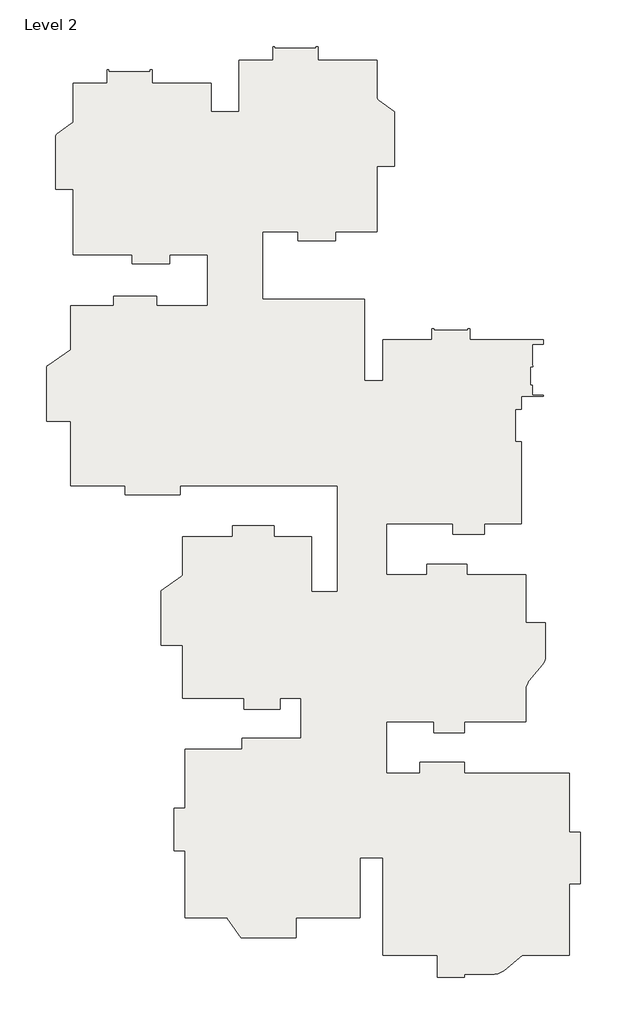
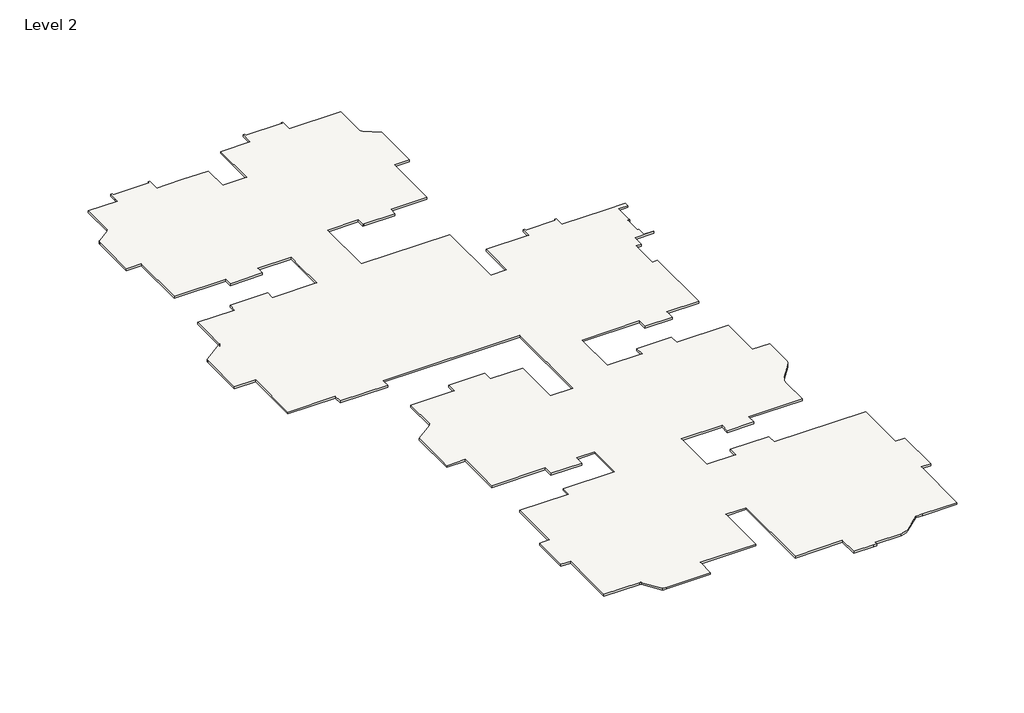
# One storey: 1 slab.
"""IFC4 building model written with IfcOpenShell, lengths in millimetres."""

from ifc_helpers import new_model, si_unit, point, frame, frame_2d, origin, place, context, project, spatial, polyline, circle_curve, trimmed, segment, composite_curve, outline, extrude, element, save

model = new_model("IFC4")

# Units and contexts
model_context = context("Model", 3, world=origin())
ifc_project = project(units=[si_unit("LENGTHUNIT", "METRE", prefix="MILLI")], contexts=[model_context])

# Site, building, storey
site = spatial("IfcSite", under=ifc_project)
building = spatial("IfcBuilding", under=site)
storey = spatial("IfcBuildingStorey", under=building, Name="Level 2", Elevation=3048.0)

# Slab
placement = place(None, origin())
element("IfcSlab", 1, ObjectType="6\" floor", at=placement, inside=storey, context=model_context, shape_type="SweptSolid", body=[
    extrude(outline(composite_curve([segment(polyline([(-9674.5009469, 28521.6416831), (-9674.5009469, 28648.2095876), (-9560.2009469, 28648.2095876), (-9560.2009469, 27756.1461172), (-8800.3399989, 27756.1461172), (-7581.1399989, 27756.1461172), (-5674.0009469, 27756.1461172), (-5674.0009469, 25878.7255084), (-3845.2009469, 25878.7255084), (-3845.2009469, 29269.6255084), (-1617.8862554, 29269.6255084), (-1617.8862554, 30161.6889788), (-1503.5862554, 30161.6889788), (-1503.5862554, 30035.1210743), (1222.0990531, 30035.1210743), (1222.0990531, 30161.6889788), (1336.3990531, 30161.6889788), (1336.3990531, 29269.6255084), (5222.5990531, 29269.6255084), (5222.5990531, 26796.9645799)]), True, "CONTINUOUS"), segment(trimmed(circle_curve(frame_2d((5425.7990531, 26796.9645799)), 203.2), [point((5222.5990531, 26796.9645799))], [point((5309.2715047, 26630.4966536))], True, "CARTESIAN"), True, "CONTINUOUS"), segment(polyline([(5309.2715047, 26630.4966536), (6365.5990531, 25891.0673698), (6365.5990531, 22297.3255084), (5222.5990531, 22297.3255084), (5222.5990531, 18017.4255084), (2479.3990531, 18017.4255084), (2479.3990531, 17431.8689406), (155.2990531, 17431.8689406), (40.9990531, 17431.8689406), (40.9990531, 18017.4255084), (-2288.081873, 18017.4255084), (-2288.081873, 13571.4182723), (4397.0990531, 13571.4182723), (4397.0990531, 8236.2461172), (5616.2990531, 8236.2461172), (5616.2990531, 10928.6450962), (8826.8620119, 10928.6450962), (8826.8620119, 11630.4346228), (8941.1620119, 11630.4346228), (8941.1620119, 11538.2450962), (11198.7752516, 11538.2450962), (11198.7752516, 11630.4346228), (11313.0752516, 11630.4346228), (11313.0752516, 10928.6450962), (14684.0990531, 10928.6450962), (16124.6398221, 10928.6450962), (16124.6398221, 10623.8450962), (15407.9990531, 10623.8450962), (15407.9990531, 9198.1565309), (15440.8254038, 9198.1565309), (15440.8254038, 9147.3565309), (15293.6990531, 9147.3565309), (15293.6990531, 7928.1565309), (15407.9990531, 7928.1565309), (15407.9990531, 7268.4875764), (16124.6398221, 7268.4875764), (16124.6398221, 7211.3375764), (14684.0990531, 7211.3375764), (14684.0990531, 6369.3461172), (14303.0990531, 6369.3461172), (14303.0990531, 5989.8129861), (14303.0990531, 4235.7461172), (14684.0990531, 4235.7461172), (14684.0990531, -1150.3497229), (12281.5704937, -1150.3497229), (12281.5704937, -1861.5497229), (10207.1414203, -1861.5497229), (10207.1414203, -1150.3497229), (5844.8990531, -1150.3497229), (5844.8990531, -4503.1497229), (8478.6664082, -4503.1497229), (8478.6664082, -3803.3538828), (11102.6990531, -3803.3538828), (11102.6990531, -4503.1497229), (14988.8990531, -4503.1497229), (14988.8990531, -7665.4497229), (16284.2990531, -7665.4497229), (16284.2990531, -9831.602777)]), True, "CONTINUOUS"), segment(trimmed(circle_curve(frame_2d((15369.8990531, -9831.602777)), 914.4), [point((16284.2990531, -9831.602777))], [point((16075.314258, -10413.4246987))], False, "CARTESIAN"), True, "CONTINUOUS"), segment(polyline([(16075.314258, -10413.4246987), (15197.8838481, -11477.2429037)]), True, "CONTINUOUS"), segment(trimmed(circle_curve(frame_2d((15903.2990531, -12059.0648255)), 914.4), [point((15197.8838481, -11477.2429037))], [point((14988.8990531, -12059.0648255))], True, "CARTESIAN"), True, "CONTINUOUS"), segment(polyline([(14988.8990531, -12059.0648255), (14988.8990531, -14167.8497229), (10937.0055378, -14167.8497229), (10937.0055378, -14879.0497229), (8943.6990531, -14879.0497229), (8943.6990531, -14167.8497229), (5844.8990531, -14167.8497229), (5844.8990531, -17520.6497229), (8028.4305674, -17520.6497229), (8028.4305674, -16809.4497229), (10950.2990531, -16809.4497229), (10950.2990531, -17520.6497229), (17846.3990531, -17520.6497229), (17846.3990531, -21406.8497229), (18557.5990531, -21406.8497229), (18557.5990531, -24797.7497229), (17846.3990531, -24797.7497229), (17846.3990531, -29484.0497229), (15255.5990531, -29484.0497229), (14750.9761043, -29484.0497229), (13536.5708908, -30485.6833283)]), True, "CONTINUOUS"), segment(trimmed(circle_curve(frame_2d((12809.2934887, -29603.9143222)), 1143.0), [point((13536.5708908, -30485.6833283))], [point((12921.9420983, -30741.3497229))], False, "CARTESIAN"), True, "CONTINUOUS"), segment(polyline([(12921.9420983, -30741.3497229), (10950.2990531, -30741.3497229), (10950.2990531, -30936.1779934), (10721.6990531, -30936.1779934), (9197.6990531, -30936.1779934), (9197.6990531, -29484.0497229), (5616.2990531, -29484.0497229), (5616.2990531, -23083.8583639), (4079.5990531, -23083.8583639), (4079.5990531, -27006.2538828), (-111.4009469, -27006.2538828), (-111.4009469, -28339.7538828), (-3426.1009469, -28339.7538828), (-3705.1428083, -28339.7538828), (-4593.0897712, -27071.2582215)]), True, "CONTINUOUS"), segment(trimmed(circle_curve(frame_2d((-4717.9407159, -27158.6538828)), 152.4), [point((-4593.0897712, -27071.2582215))], [point((-4717.9407159, -27006.2538828))], True, "CARTESIAN"), True, "CONTINUOUS"), segment(polyline([(-4717.9407159, -27006.2538828), (-7388.5009469, -27006.2538828), (-7388.5009469, -22629.8863256), (-8112.4009469, -22629.8863256), (-8112.4009469, -19843.4538828), (-7388.5009469, -19843.4538828), (-7388.5009469, -15957.2538828), (-3654.7009469, -15957.2538828), (-3654.7009469, -15233.3538828), (231.4990531, -15233.3538828), (231.4990531, -12604.4538828), (-1152.8009469, -12604.4538828), (-1152.8009469, -13328.3538828), (-3515.0009469, -13328.3538828), (-3515.0009469, -12604.4538828), (-7553.6009469, -12604.4538828), (-7553.6009469, -9137.3538828), (-8963.3009469, -9137.3538828), (-8963.3009469, -5543.6120214), (-7618.6052856, -4602.3250585)]), True, "CONTINUOUS"), segment(trimmed(circle_curve(frame_2d((-7706.0009469, -4477.4741138)), 152.4), [point((-7618.6052856, -4602.3250585))], [point((-7553.6009469, -4477.4741138))], True, "CARTESIAN"), True, "CONTINUOUS"), segment(polyline([(-7553.6009469, -4477.4741138), (-7553.6009469, -2012.6538828), (-4277.0009469, -2012.6538828), (-4277.0009469, -1288.7538828), (-1533.8009469, -1288.7538828), (-1533.8009469, -2012.6538828), (904.5990531, -2012.6538828), (904.5990531, -5632.1538828), (2631.7990531, -5632.1538828), (2631.7990531, 1340.1461172), (-7726.7333092, 1340.1461172), (-7726.7333092, 730.5461172), (-11312.8009469, 730.5461172), (-11312.8009469, 1340.1461172), (-14894.2009469, 1340.1461172), (-14894.2009469, 5569.2461172), (-16494.4009469, 5569.2461172), (-16494.4009469, 9057.1907685)]), True, "CONTINUOUS"), segment(trimmed(circle_curve(frame_2d((-16291.2009469, 9057.1907685)), 203.2), [point((-16494.4009469, 9057.1907685))], [point((-16407.7284953, 9223.6586947))], False, "CARTESIAN"), True, "CONTINUOUS"), segment(polyline([(-16407.7284953, 9223.6586947), (-14915.8690598, 10267.9602996)]), True, "CONTINUOUS"), segment(trimmed(circle_curve(frame_2d((-14945.0009469, 10309.5772811)), 50.8), [point((-14915.8690598, 10267.9602996))], [point((-14894.2009469, 10309.5772811))], True, "CARTESIAN"), True, "CONTINUOUS"), segment(polyline([(-14894.2009469, 10309.5772811), (-14894.2009469, 13151.1461172), (-12085.9698258, 13151.1461172), (-12085.9698258, 13760.7461172), (-9255.4009469, 13760.7461172), (-9255.4009469, 13151.1461172), (-5902.6009469, 13151.1461172), (-5902.6009469, 15437.1461172), (-5902.6009469, 16503.9461172), (-8417.2009469, 16503.9461172), (-8417.2009469, 15918.3895495), (-10855.6009469, 15918.3895495), (-10855.6009469, 16503.9461172), (-14741.8009469, 16503.9461172), (-14741.8009469, 20783.8461172), (-15884.8009469, 20783.8461172), (-15884.8009469, 24271.7907685)]), True, "CONTINUOUS"), segment(trimmed(circle_curve(frame_2d((-15681.6009469, 24271.7907685)), 203.2), [point((-15884.8009469, 24271.7907685))], [point((-15798.1284953, 24438.2586947))], False, "CARTESIAN"), True, "CONTINUOUS"), segment(polyline([(-15798.1284953, 24438.2586947), (-14828.4733986, 25117.0172625)]), True, "CONTINUOUS"), segment(trimmed(circle_curve(frame_2d((-14945.0009469, 25283.4851887)), 203.2), [point((-14828.4733986, 25117.0172625))], [point((-14741.8009469, 25283.4851887))], True, "CARTESIAN"), True, "CONTINUOUS"), segment(polyline([(-14741.8009469, 25283.4851887), (-14741.8009469, 27756.1461172), (-12514.4862554, 27756.1461172), (-12514.4862554, 28060.9461172), (-12514.4862554, 28648.2095876), (-12400.1862554, 28648.2095876), (-12400.1862554, 28521.6416831), (-9674.5009469, 28521.6416831)]), True, "CONTINUOUS")], self_intersect=False)), frame((0.0, 0.0, 3048.0), z_axis=(0.0, 0.0, 1.0), x_axis=(1.0, 0.0, 0.0)), (0.0, 0.0, 1.0), 152.4),
])

save(model, "model.ifc")

# Revit data of these elements
# Type "6\" floor"
#   Assembly Code = "B1010"
#   Function = 0
#   Layers, outside or top first: 0' - 6" no material (function 1)
# Element 1 (IfcSlab, "6\" floor")
#   Height Offset From Level = 0' - 6"
#   Phase Created = New Construction
#   Materials on its faces: "Default Floor"
# Materials
#   "Default Floor": colour RGB 128 128 128, transparency 0, Cost = 0
